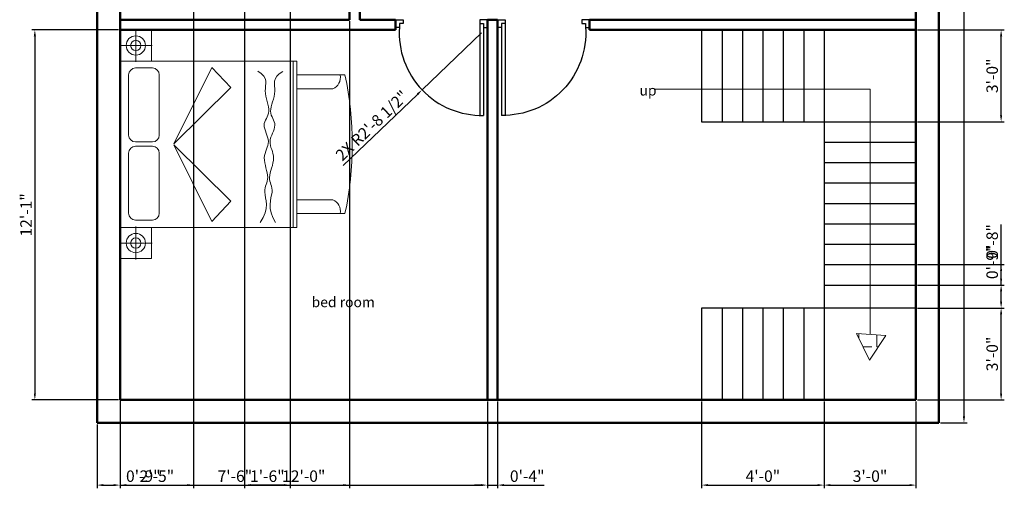
# Model space of a CAD drawing. Units: inches. Extents: x 1253 to 1645, y 2180 to 2698.
# Tile 1 of 5: x 1257 to 1643, y 2180 to 2363. Entities that reach past the tile are written whole.
import ezdxf

# ---------------------------------------------------------------- set-up
doc = ezdxf.new("R2010")
doc.units = ezdxf.units.IN
for name, color, linetype, lineweight in [('A-ANNO-DIMS', 2, 'Continuous', 18), ('A-ANNO-SYMB', 7, 'Continuous', 18), ('A-ANNO-TEXT', 7, 'Continuous', 18), ('A-AREA-IDEN', 7, 'Continuous', 25), ('A-DOOR', 4, 'Continuous', 25), ('A-FLOR-STRS', 7, 'Continuous', 25), ('A-FURN', 8, 'Continuous', 18), ('wall', 7, 'Continuous', 50)]:
    doc.layers.add(name, color=color, linetype=linetype, lineweight=lineweight)
doc.styles.get("Standard").update_dxf_attribs({"font": 'arial.ttf'})
doc.dimstyles.new('ISO-25', dxfattribs={"dimtxt": 4.5, "dimasz": 2.5, "dimexe": 1.25, "dimexo": 0.625, "dimtad": 1, "dimdec": 1, "dimlunit": 3, "dimtxsty": 'Standard', "dimcen": 4.5, "dimadec": 0, "dimazin": 0, "dimtfac": 1, "dimtdec": 1, "dimtmove": 0, "dimatfit": 3, "dimfxl": 1, "dimarcsym": 0})

# ---------------------------------------------------------------- blocks, each defined once
blk = doc.blocks.new('A$C4F543DC7')
for p, q in [((0.013, 3.35, -0.169), (3.313, 3.35, -0.169)), ((0.463, 3.35, -0.169), (0.013, 3.35, -0.169)), ((0.013, 2.896, -0.169), (0.013, 3.35, -0.169)), ((0.013, 3.35, -0.169), (0.013, 2.896, -0.169)), ((0.238, 3.123, -0.439), (0.238, 3.361, -0.439)), ((0.463, 3.35, -0.169), (0.463, 0.8, -0.169)), ((2.863, 3.35, -0.169), (0.463, 3.35, -0.169)), ((0.463, 2.896, -0.169), (0.463, 3.35, -0.169)), ((2.863, 0.8, -0.169), (2.863, 3.35, -0.169)), ((2.863, 3.35, -0.169), (3.313, 3.35, -0.169)), ((2.863, 2.896, -0.169), (2.863, 3.35, -0.169)), ((3.089, 3.123, -0.439), (3.089, 3.361, -0.439)), ((3.313, 3.35, -0.169), (3.313, 2.896, -0.169)), ((3.313, 3.35, -0.169), (3.313, 2.896, -0.169)), ((1.535, 3.226, -0.169), (0.668, 3.226, -0.169)), ((2.664, 3.226, -0.169), (1.797, 3.226, -0.169)), ((0.238, 3.123, -0.439), (0, 3.123, -0.439)), ((0.238, 3.123, -0.439), (0.476, 3.123, -0.439)), ((0.238, 3.123, -0.439), (0.238, 2.885, -0.439)), ((0.568, 3.126, -0.169), (0.568, 2.884, -0.169)), ((1.635, 2.884, -0.169), (1.635, 3.126, -0.169)), ((1.697, 3.126, -0.169), (1.697, 2.884, -0.169)), ((2.764, 2.884, -0.169), (2.764, 3.126, -0.169)), ((3.089, 3.123, -0.439), (2.851, 3.123, -0.439)), ((3.089, 3.123, -0.439), (3.089, 2.885, -0.439)), ((3.089, 3.123, -0.439), (3.327, 3.123, -0.439)), ((0.463, 2.896, -0.169), (0.013, 2.896, -0.169)), ((0.013, 2.896, -0.169), (0.463, 2.896, -0.169)), ((0.463, 0.8, -0.169), (0.463, 2.896, -0.169)), ((2.863, 2.896, -0.169), (2.863, 0.8, -0.169)), ((3.313, 2.896, -0.169), (2.863, 2.896, -0.169)), ((3.313, 2.896, -0.169), (2.863, 2.896, -0.169)), ((0.668, 2.784, -0.169), (1.535, 2.784, -0.169)), ((1.797, 2.784, -0.169), (2.664, 2.784, -0.169)), ((1.653, 2.573, -0.169), (0.55, 2.025, -0.169)), ((0.841, 1.752, -0.169), (1.653, 2.573, -0.169)), ((2.481, 1.752, -0.169), (1.669, 2.573, -0.169)), ((1.669, 2.573, -0.169), (2.772, 2.025, -0.169)), ((0.55, 2.025, -0.169), (0.841, 1.752, -0.169)), ((2.772, 2.025, -0.169), (2.481, 1.752, -0.169)), ((0.537, 1.327, -0.169), (0.609, 1.284, -0.169)), ((0.609, 1.284, -0.169), (0.676, 1.257, -0.169)), ((2.648, 1.277, -0.169), (2.683, 1.312, -0.169)), ((2.683, 1.312, -0.169), (2.718, 1.364, -0.169)), ((0.533, 1.105, -0.169), (0.607, 1.146, -0.169)), ((0.607, 1.146, -0.169), (0.674, 1.171, -0.169)), ((0.674, 1.171, -0.169), (0.736, 1.183, -0.169)), ((0.676, 1.257, -0.169), (0.737, 1.243, -0.169)), ((0.736, 1.183, -0.169), (0.793, 1.185, -0.169)), ((0.737, 1.243, -0.169), (0.794, 1.239, -0.169)), ((0.793, 1.185, -0.169), (0.845, 1.18, -0.169)), ((0.794, 1.239, -0.169), (0.846, 1.242, -0.169)), ((0.845, 1.18, -0.169), (0.891, 1.172, -0.169)), ((0.846, 1.242, -0.169), (0.893, 1.249, -0.169)), ((0.891, 1.172, -0.169), (0.933, 1.163, -0.169)), ((0.893, 1.249, -0.169), (0.935, 1.256, -0.169)), ((0.933, 1.163, -0.169), (0.97, 1.156, -0.169)), ((0.935, 1.256, -0.169), (0.972, 1.261, -0.169)), ((0.97, 1.156, -0.169), (1.003, 1.155, -0.169)), ((0.972, 1.261, -0.169), (1.004, 1.262, -0.169)), ((1.003, 1.155, -0.169), (1.032, 1.158, -0.169)), ((1.004, 1.262, -0.169), (1.033, 1.258, -0.169)), ((1.032, 1.158, -0.169), (1.058, 1.164, -0.169)), ((1.033, 1.258, -0.169), (1.06, 1.251, -0.169)), ((1.058, 1.164, -0.169), (1.083, 1.172, -0.169)), ((1.06, 1.251, -0.169), (1.084, 1.242, -0.169)), ((1.083, 1.172, -0.169), (1.107, 1.18, -0.169)), ((1.084, 1.242, -0.169), (1.108, 1.234, -0.169)), ((1.107, 1.18, -0.169), (1.132, 1.187, -0.169)), ((1.108, 1.234, -0.169), (1.132, 1.226, -0.169)), ((1.132, 1.226, -0.169), (1.158, 1.22, -0.169)), ((1.132, 1.187, -0.169), (1.157, 1.192, -0.169)), ((1.157, 1.192, -0.169), (1.185, 1.193, -0.169)), ((1.158, 1.22, -0.169), (1.185, 1.218, -0.169)), ((1.185, 1.218, -0.169), (1.216, 1.22, -0.169)), ((1.185, 1.193, -0.169), (1.216, 1.19, -0.169)), ((1.216, 1.22, -0.169), (1.25, 1.226, -0.169)), ((1.216, 1.19, -0.169), (1.249, 1.183, -0.169)), ((1.249, 1.183, -0.169), (1.284, 1.173, -0.169)), ((1.25, 1.226, -0.169), (1.285, 1.235, -0.169)), ((1.284, 1.173, -0.169), (1.321, 1.163, -0.169)), ((1.285, 1.235, -0.169), (1.322, 1.244, -0.169)), ((1.321, 1.163, -0.169), (1.358, 1.152, -0.169)), ((1.322, 1.244, -0.169), (1.359, 1.253, -0.169)), ((1.358, 1.152, -0.169), (1.394, 1.143, -0.169)), ((1.359, 1.253, -0.169), (1.396, 1.261, -0.169)), ((1.394, 1.143, -0.169), (1.431, 1.137, -0.169)), ((1.396, 1.261, -0.169), (1.433, 1.266, -0.169)), ((1.431, 1.137, -0.169), (1.466, 1.135, -0.169)), ((1.433, 1.266, -0.169), (1.468, 1.268, -0.169)), ((1.466, 1.135, -0.169), (1.499, 1.137, -0.169)), ((1.468, 1.268, -0.169), (1.501, 1.264, -0.169)), ((1.499, 1.137, -0.169), (1.531, 1.143, -0.169)), ((1.501, 1.264, -0.169), (1.532, 1.257, -0.169)), ((1.531, 1.143, -0.169), (1.561, 1.152, -0.169)), ((1.532, 1.257, -0.169), (1.562, 1.247, -0.169)), ((1.561, 1.152, -0.169), (1.59, 1.162, -0.169)), ((1.562, 1.247, -0.169), (1.591, 1.237, -0.169)), ((1.59, 1.162, -0.169), (1.619, 1.172, -0.169)), ((1.591, 1.237, -0.169), (1.62, 1.226, -0.169)), ((1.619, 1.172, -0.169), (1.648, 1.18, -0.169)), ((1.62, 1.226, -0.169), (1.648, 1.217, -0.169)), ((1.648, 1.217, -0.169), (1.676, 1.211, -0.169)), ((1.648, 1.18, -0.169), (1.676, 1.185, -0.169)), ((1.676, 1.211, -0.169), (1.705, 1.209, -0.169)), ((1.676, 1.185, -0.169), (1.705, 1.186, -0.169)), ((1.705, 1.209, -0.169), (1.735, 1.212, -0.169)), ((1.705, 1.186, -0.169), (1.734, 1.182, -0.169)), ((1.734, 1.182, -0.169), (1.764, 1.173, -0.169)), ((1.735, 1.212, -0.169), (1.765, 1.22, -0.169)), ((1.764, 1.173, -0.169), (1.794, 1.162, -0.169)), ((1.765, 1.22, -0.169), (1.795, 1.23, -0.169)), ((1.794, 1.162, -0.169), (1.824, 1.149, -0.169)), ((1.795, 1.23, -0.169), (1.826, 1.242, -0.169)), ((1.824, 1.149, -0.169), (1.854, 1.137, -0.169)), ((1.826, 1.242, -0.169), (1.856, 1.253, -0.169)), ((1.854, 1.137, -0.169), (1.883, 1.126, -0.169)), ((1.856, 1.253, -0.169), (1.885, 1.263, -0.169)), ((1.885, 1.263, -0.169), (1.913, 1.27, -0.169)), ((1.913, 1.27, -0.169), (1.94, 1.272, -0.169)), ((1.94, 1.272, -0.169), (1.965, 1.269, -0.169)), ((1.965, 1.269, -0.169), (1.989, 1.262, -0.169)), ((1.989, 1.262, -0.169), (2.012, 1.251, -0.169)), ((2.011, 1.134, -0.169), (2.034, 1.145, -0.169)), ((2.012, 1.251, -0.169), (2.036, 1.239, -0.169)), ((2.034, 1.145, -0.169), (2.059, 1.157, -0.169)), ((2.036, 1.239, -0.169), (2.06, 1.227, -0.169)), ((2.059, 1.157, -0.169), (2.084, 1.167, -0.169)), ((2.06, 1.227, -0.169), (2.085, 1.216, -0.169)), ((2.084, 1.167, -0.169), (2.111, 1.174, -0.169)), ((2.085, 1.216, -0.169), (2.112, 1.208, -0.169)), ((2.111, 1.174, -0.169), (2.14, 1.177, -0.169)), ((2.112, 1.208, -0.169), (2.141, 1.204, -0.169)), ((2.14, 1.177, -0.169), (2.172, 1.175, -0.169)), ((2.141, 1.204, -0.169), (2.172, 1.205, -0.169)), ((2.172, 1.205, -0.169), (2.206, 1.21, -0.169)), ((2.172, 1.175, -0.169), (2.206, 1.169, -0.169)), ((2.206, 1.21, -0.169), (2.242, 1.218, -0.169)), ((2.206, 1.169, -0.169), (2.241, 1.16, -0.169)), ((2.241, 1.16, -0.169), (2.278, 1.149, -0.169)), ((2.242, 1.218, -0.169), (2.279, 1.228, -0.169)), ((2.278, 1.149, -0.169), (2.316, 1.138, -0.169)), ((2.279, 1.228, -0.169), (2.317, 1.238, -0.169)), ((2.316, 1.138, -0.169), (2.354, 1.128, -0.169)), ((2.317, 1.238, -0.169), (2.356, 1.246, -0.169)), ((2.356, 1.246, -0.169), (2.394, 1.253, -0.169)), ((2.394, 1.253, -0.169), (2.433, 1.255, -0.169)), ((2.433, 1.255, -0.169), (2.47, 1.253, -0.169)), ((2.47, 1.253, -0.169), (2.506, 1.249, -0.169)), ((2.506, 1.249, -0.169), (2.542, 1.246, -0.169)), ((2.542, 1.246, -0.169), (2.578, 1.248, -0.169)), ((2.578, 1.248, -0.169), (2.613, 1.257, -0.169)), ((2.613, 1.257, -0.169), (2.648, 1.277, -0.169)), ((1.883, 1.126, -0.169), (1.911, 1.119, -0.169)), ((1.911, 1.119, -0.169), (1.937, 1.115, -0.169)), ((1.937, 1.115, -0.169), (1.963, 1.118, -0.169)), ((1.963, 1.118, -0.169), (1.987, 1.124, -0.169)), ((1.987, 1.124, -0.169), (2.011, 1.134, -0.169)), ((2.354, 1.128, -0.169), (2.392, 1.121, -0.169)), ((2.392, 1.121, -0.169), (2.43, 1.117, -0.169)), ((2.43, 1.117, -0.169), (2.468, 1.118, -0.169)), ((2.468, 1.118, -0.169), (2.504, 1.121, -0.169)), ((2.504, 1.121, -0.169), (2.54, 1.123, -0.169)), ((2.54, 1.123, -0.169), (2.576, 1.12, -0.169)), ((2.576, 1.12, -0.169), (2.611, 1.109, -0.169)), ((2.611, 1.109, -0.169), (2.645, 1.088, -0.169)), ((2.645, 1.088, -0.169), (2.679, 1.052, -0.169)), ((2.679, 1.052, -0.169), (2.712, 0.999, -0.169)), ((0.463, 0.85, -0.169), (2.863, 0.85, -0.169)), ((0.463, 0.8, -0.169), (2.863, 0.8, -0.169)), ((0.663, 0.8, -0.169), (0.463, 0.8, -0.169)), ((0.663, 0.8, -0.169), (2.663, 0.8, -0.169)), ((0.663, 0.104, -0.169), (0.663, 0.8, -0.169)), ((0.663, 0.104, -0.169), (0.663, 0.8, -0.169)), ((0.863, 0.281, -0.169), (0.863, 0.8, -0.169)), ((2.463, 0.8, -0.169), (2.463, 0.281, -0.169)), ((2.863, 0.8, -0.169), (2.663, 0.8, -0.169)), ((2.663, 0.8, -0.169), (2.663, 0.104, -0.169)), ((2.663, 0.8, -0.169), (2.663, 0.104, -0.169))]:
    blk.add_line(p, q)
for centre, radius in [((0.238, 3.123, -0.439), 0.139), ((0.238, 3.123, -0.439), 0.075), ((3.089, 3.123, -0.439), 0.139), ((3.089, 3.123, -0.439), 0.075)]:
    blk.add_circle(centre, radius)
for centre, radius, start, end in [((0.668, 3.126, -0.169), 0.1, 90, 180), ((1.535, 3.126, -0.169), 0.1, 0, 90), ((1.797, 3.126, -0.169), 0.1, 90, 180), ((2.664, 3.126, -0.169), 0.1, 0, 90), ((0.668, 2.884, -0.169), 0.1, 180, 270), ((1.535, 2.884, -0.169), 0.1, 270, 0), ((1.797, 2.884, -0.169), 0.1, 180, 270), ((2.664, 2.884, -0.169), 0.1, 270, 0), ((0.699, 0.347, -0.169), 0.177, 258.2616, 338.032), ((2.627, 0.347, -0.169), 0.177, 201.968, 281.7384), ((1.663, 4.86, -0.169), 4.86, 258.1252, 281.8748), ((1.663, 4.86, -0.169), 4.86, 258.1252, 281.8748)]:
    blk.add_arc(centre, radius, start, end)
blk = doc.blocks.new('*D14')
at = {"layer": 'A-ANNO-DIMS', "color": 0, "lineweight": -2, "transparency": 16777216}
for p, q in [((1617.57, 2667.35), (1628.02, 2667.35)), ((1626.77, 2664.85), (1626.77, 2207.85)), ((1617.57, 2205.35), (1628.02, 2205.35))]:
    blk.add_line(p, q, dxfattribs=at)
at = {"layer": 'A-ANNO-DIMS', "color": 0, "transparency": 16777216}
for points in [[(1626.36, 2664.85), (1627.19, 2664.85), (1626.77, 2667.35)], [(1626.36, 2207.85), (1627.19, 2207.85), (1626.77, 2205.35)]]:
    blk.add_solid(points, dxfattribs=at)
at = {"layer": 'Defpoints', "color": 0, "transparency": 16777216}
for p in [(1616.94, 2667.35), (1616.94, 2205.35), (1626.77, 2205.35)]:
    blk.add_point(p, dxfattribs=at)
at = {"layer": 'A-ANNO-DIMS', "color": 0, "transparency": 16777216, "insert": (1623.85, 2436.35), "char_height": 4.5, "attachment_point": 5, "rotation": 90}
blk.add_mtext('38\'-6"', dxfattribs=at)
blk = doc.blocks.new('DOOR-SWING-36IN')
for p, q in [((1.5, 1.5), (1.5, 37.5)), ((3, 1.5), (3, 37.5)), ((0, 3), (0, 0)), ((1.5, 3), (0, 3)), ((1.5, 1.5), (1.5, 3)), ((3, 1.5), (1.5, 1.5)), ((3, 0), (3, 1.5)), ((33, 0), (33, 1.5)), ((33, 1.5), (34.5, 1.5)), ((34.5, 1.5), (34.5, 3)), ((34.5, 3), (36, 3)), ((36, 3), (36, 0)), ((0, 0), (3, 0)), ((36, 0), (33, 0))]:
    blk.add_line(p, q)
blk.add_arc((2.25, 5.18), 32.32, 356.1244, 91.3295)
blk = doc.blocks.new('*D33')
at = {"layer": 'A-ANNO-DIMS', "color": 0, "lineweight": -2, "transparency": 16777216}
for p, q in [((1295.32, 2359.35), (1261.29, 2359.35)), ((1262.54, 2356.85), (1262.54, 2216.85)), ((1295.32, 2214.35), (1261.29, 2214.35))]:
    blk.add_line(p, q, dxfattribs=at)
at = {"layer": 'A-ANNO-DIMS', "color": 0, "transparency": 16777216}
for points in [[(1262.12, 2356.85), (1262.96, 2356.85), (1262.54, 2359.35)], [(1262.12, 2216.85), (1262.96, 2216.85), (1262.54, 2214.35)]]:
    blk.add_solid(points, dxfattribs=at)
at = {"layer": 'Defpoints', "color": 0, "transparency": 16777216}
for p in [(1295.94, 2359.35), (1262.54, 2214.35), (1295.94, 2214.35)]:
    blk.add_point(p, dxfattribs=at)
at = {"layer": 'A-ANNO-DIMS', "color": 0, "transparency": 16777216, "insert": (1259.66, 2286.85), "char_height": 4.5, "attachment_point": 5, "rotation": 90}
blk.add_mtext('12\'-1"', dxfattribs=at)
blk = doc.blocks.new('*D34')
at = {"layer": 'A-ANNO-DIMS', "color": 0, "lineweight": -2, "transparency": 16777216}
for p, q in [((1295.94, 2213.72), (1295.94, 2179.7)), ((1439.94, 2213.72), (1439.94, 2179.7)), ((1298.44, 2180.95), (1437.44, 2180.95))]:
    blk.add_line(p, q, dxfattribs=at)
at = {"layer": 'A-ANNO-DIMS', "color": 0, "transparency": 16777216}
for points in [[(1298.44, 2181.36), (1298.44, 2180.53), (1295.94, 2180.95)], [(1437.44, 2181.36), (1437.44, 2180.53), (1439.94, 2180.95)]]:
    blk.add_solid(points, dxfattribs=at)
at = {"layer": 'Defpoints', "color": 0, "transparency": 16777216}
for p in [(1295.94, 2214.35), (1439.94, 2214.35), (1439.94, 2180.95)]:
    blk.add_point(p, dxfattribs=at)
at = {"layer": 'A-ANNO-DIMS', "color": 0, "transparency": 16777216, "insert": (1367.94, 2183.87), "char_height": 4.5, "attachment_point": 5}
blk.add_mtext('12\'-0"', dxfattribs=at)
blk = doc.blocks.new('*D35')
at = {"layer": 'A-ANNO-DIMS', "color": 0, "lineweight": -2, "transparency": 16777216}
for p, q in [((1295.94, 2362.72), (1295.94, 2179.7)), ((1385.94, 2362.72), (1385.94, 2179.7)), ((1298.44, 2180.95), (1383.44, 2180.95))]:
    blk.add_line(p, q, dxfattribs=at)
at = {"layer": 'A-ANNO-DIMS', "color": 0, "transparency": 16777216}
for points in [[(1298.44, 2181.36), (1298.44, 2180.53), (1295.94, 2180.95)], [(1383.44, 2181.36), (1383.44, 2180.53), (1385.94, 2180.95)]]:
    blk.add_solid(points, dxfattribs=at)
at = {"layer": 'Defpoints', "color": 0, "transparency": 16777216}
for p in [(1295.94, 2363.35), (1385.94, 2363.35), (1385.94, 2180.95)]:
    blk.add_point(p, dxfattribs=at)
at = {"layer": 'A-ANNO-DIMS', "color": 0, "transparency": 16777216, "insert": (1340.94, 2183.87), "char_height": 4.5, "attachment_point": 5}
blk.add_mtext('7\'-6"', dxfattribs=at)
blk = doc.blocks.new('*D36')
at = {"layer": 'A-ANNO-DIMS', "color": 0, "lineweight": -2, "transparency": 16777216}
for p, q in [((1523.94, 2213.72), (1523.94, 2179.7)), ((1571.94, 2213.72), (1571.94, 2179.7)), ((1526.44, 2180.95), (1569.44, 2180.95))]:
    blk.add_line(p, q, dxfattribs=at)
at = {"layer": 'A-ANNO-DIMS', "color": 0, "transparency": 16777216}
for points in [[(1526.44, 2181.36), (1526.44, 2180.53), (1523.94, 2180.95)], [(1569.44, 2181.36), (1569.44, 2180.53), (1571.94, 2180.95)]]:
    blk.add_solid(points, dxfattribs=at)
at = {"layer": 'Defpoints', "color": 0, "transparency": 16777216}
for p in [(1523.94, 2214.35), (1571.94, 2214.35), (1571.94, 2180.95)]:
    blk.add_point(p, dxfattribs=at)
at = {"layer": 'A-ANNO-DIMS', "color": 0, "transparency": 16777216, "insert": (1547.94, 2183.87), "char_height": 4.5, "attachment_point": 5}
blk.add_mtext('4\'-0"', dxfattribs=at)
blk = doc.blocks.new('*D37')
at = {"layer": 'A-ANNO-DIMS', "color": 0, "lineweight": -2, "transparency": 16777216}
for p, q in [((1571.94, 2213.72), (1571.94, 2179.7)), ((1607.94, 2213.72), (1607.94, 2179.7)), ((1574.44, 2180.95), (1605.44, 2180.95))]:
    blk.add_line(p, q, dxfattribs=at)
at = {"layer": 'A-ANNO-DIMS', "color": 0, "transparency": 16777216}
for points in [[(1574.44, 2181.36), (1574.44, 2180.53), (1571.94, 2180.95)], [(1605.44, 2181.36), (1605.44, 2180.53), (1607.94, 2180.95)]]:
    blk.add_solid(points, dxfattribs=at)
at = {"layer": 'Defpoints', "color": 0, "transparency": 16777216}
for p in [(1571.94, 2214.35), (1607.94, 2214.35), (1607.94, 2180.95)]:
    blk.add_point(p, dxfattribs=at)
at = {"layer": 'A-ANNO-DIMS', "color": 0, "transparency": 16777216, "insert": (1589.94, 2183.87), "char_height": 4.5, "attachment_point": 5}
blk.add_mtext('3\'-0"', dxfattribs=at)
blk = doc.blocks.new('*D38')
at = {"layer": 'A-ANNO-DIMS', "color": 0, "lineweight": -2, "transparency": 16777216}
for p, q in [((1641.34, 2259.35), (1641.34, 2275.06)), ((1608.57, 2259.35), (1642.59, 2259.35)), ((1641.34, 2252.85), (1641.34, 2256.85)), ((1608.57, 2250.35), (1642.59, 2250.35))]:
    blk.add_line(p, q, dxfattribs=at)
at = {"layer": 'A-ANNO-DIMS', "color": 0, "transparency": 16777216}
for points in [[(1640.92, 2256.85), (1641.76, 2256.85), (1641.34, 2259.35)], [(1640.92, 2252.85), (1641.76, 2252.85), (1641.34, 2250.35)]]:
    blk.add_solid(points, dxfattribs=at)
at = {"layer": 'Defpoints', "color": 0, "transparency": 16777216}
for p in [(1607.94, 2259.35), (1641.34, 2259.35), (1607.94, 2250.35)]:
    blk.add_point(p, dxfattribs=at)
at = {"layer": 'A-ANNO-DIMS', "color": 0, "transparency": 16777216, "insert": (1638.42, 2268.45), "char_height": 4.5, "attachment_point": 5, "rotation": 90}
blk.add_mtext('0\'-9"', dxfattribs=at)
blk = doc.blocks.new('*D39')
at = {"layer": 'A-ANNO-DIMS', "color": 0, "lineweight": -2, "transparency": 16777216}
for p, q in [((1641.34, 2267.35), (1641.34, 2283.06)), ((1608.57, 2267.35), (1642.59, 2267.35)), ((1641.34, 2261.85), (1641.34, 2264.85)), ((1608.57, 2259.35), (1642.59, 2259.35))]:
    blk.add_line(p, q, dxfattribs=at)
at = {"layer": 'A-ANNO-DIMS', "color": 0, "transparency": 16777216}
for points in [[(1640.92, 2264.85), (1641.76, 2264.85), (1641.34, 2267.35)], [(1640.92, 2261.85), (1641.76, 2261.85), (1641.34, 2259.35)]]:
    blk.add_solid(points, dxfattribs=at)
at = {"layer": 'Defpoints', "color": 0, "transparency": 16777216}
for p in [(1607.94, 2267.35), (1641.34, 2267.35), (1607.94, 2259.35)]:
    blk.add_point(p, dxfattribs=at)
at = {"layer": 'A-ANNO-DIMS', "color": 0, "transparency": 16777216, "insert": (1638.42, 2276.45), "char_height": 4.5, "attachment_point": 5, "rotation": 90}
blk.add_mtext('0\'-8"', dxfattribs=at)
blk = doc.blocks.new('*D40')
at = {"layer": 'A-ANNO-DIMS', "color": 0, "lineweight": -2, "transparency": 16777216}
for p, q in [((1608.57, 2359.35), (1642.59, 2359.35)), ((1641.34, 2325.85), (1641.34, 2356.85)), ((1608.57, 2323.35), (1642.59, 2323.35))]:
    blk.add_line(p, q, dxfattribs=at)
at = {"layer": 'A-ANNO-DIMS', "color": 0, "transparency": 16777216}
for points in [[(1640.92, 2356.85), (1641.76, 2356.85), (1641.34, 2359.35)], [(1640.92, 2325.85), (1641.76, 2325.85), (1641.34, 2323.35)]]:
    blk.add_solid(points, dxfattribs=at)
at = {"layer": 'Defpoints', "color": 0, "transparency": 16777216}
for p in [(1607.94, 2359.35), (1641.34, 2359.35), (1607.94, 2323.35)]:
    blk.add_point(p, dxfattribs=at)
at = {"layer": 'A-ANNO-DIMS', "color": 0, "transparency": 16777216, "insert": (1638.42, 2341.35), "char_height": 4.5, "attachment_point": 5, "rotation": 90}
blk.add_mtext('3\'-0"', dxfattribs=at)
blk = doc.blocks.new('*D41')
at = {"layer": 'A-ANNO-DIMS', "color": 0, "lineweight": -2, "transparency": 16777216}
for p, q in [((1608.57, 2250.35), (1642.59, 2250.35)), ((1641.34, 2216.85), (1641.34, 2247.85)), ((1608.57, 2214.35), (1642.59, 2214.35))]:
    blk.add_line(p, q, dxfattribs=at)
at = {"layer": 'A-ANNO-DIMS', "color": 0, "transparency": 16777216}
for points in [[(1640.92, 2247.85), (1641.76, 2247.85), (1641.34, 2250.35)], [(1640.92, 2216.85), (1641.76, 2216.85), (1641.34, 2214.35)]]:
    blk.add_solid(points, dxfattribs=at)
at = {"layer": 'Defpoints', "color": 0, "transparency": 16777216}
for p in [(1607.94, 2250.35), (1641.34, 2250.35), (1607.94, 2214.35)]:
    blk.add_point(p, dxfattribs=at)
at = {"layer": 'A-ANNO-DIMS', "color": 0, "transparency": 16777216, "insert": (1638.42, 2232.35), "char_height": 4.5, "attachment_point": 5, "rotation": 90}
blk.add_mtext('3\'-0"', dxfattribs=at)
blk = doc.blocks.new('*D42')
at = {"layer": 'A-ANNO-DIMS', "color": 0, "lineweight": -2, "transparency": 16777216}
for p, q in [((1295.94, 2213.72), (1295.94, 2179.7)), ((1286.94, 2204.72), (1286.94, 2179.7)), ((1289.44, 2180.95), (1293.44, 2180.95)), ((1295.94, 2180.95), (1311.65, 2180.95))]:
    blk.add_line(p, q, dxfattribs=at)
at = {"layer": 'A-ANNO-DIMS', "color": 0, "transparency": 16777216}
for points in [[(1289.44, 2181.36), (1289.44, 2180.53), (1286.94, 2180.95)], [(1293.44, 2181.36), (1293.44, 2180.53), (1295.94, 2180.95)]]:
    blk.add_solid(points, dxfattribs=at)
at = {"layer": 'Defpoints', "color": 0, "transparency": 16777216}
for p in [(1295.94, 2214.35), (1286.94, 2205.35), (1295.94, 2180.95)]:
    blk.add_point(p, dxfattribs=at)
at = {"layer": 'A-ANNO-DIMS', "color": 0, "transparency": 16777216, "insert": (1305.05, 2183.87), "char_height": 4.5, "attachment_point": 5}
blk.add_mtext('0\'-9"', dxfattribs=at)
blk = doc.blocks.new('*D43')
at = {"layer": 'A-ANNO-DIMS', "color": 0, "lineweight": -2, "transparency": 16777216}
for p, q in [((1439.94, 2213.72), (1439.94, 2179.7)), ((1443.94, 2213.72), (1443.94, 2179.7)), ((1437.44, 2180.95), (1434.94, 2180.95)), ((1439.94, 2180.95), (1443.94, 2180.95)), ((1446.44, 2180.95), (1462.15, 2180.95))]:
    blk.add_line(p, q, dxfattribs=at)
at = {"layer": 'A-ANNO-DIMS', "color": 0, "transparency": 16777216}
for points in [[(1437.44, 2181.36), (1437.44, 2180.53), (1439.94, 2180.95)], [(1446.44, 2181.36), (1446.44, 2180.53), (1443.94, 2180.95)]]:
    blk.add_solid(points, dxfattribs=at)
at = {"layer": 'Defpoints', "color": 0, "transparency": 16777216}
for p in [(1439.94, 2214.35), (1443.94, 2214.35), (1443.94, 2180.95)]:
    blk.add_point(p, dxfattribs=at)
at = {"layer": 'A-ANNO-DIMS', "color": 0, "transparency": 16777216, "insert": (1455.55, 2183.87), "char_height": 4.5, "attachment_point": 5}
blk.add_mtext('0\'-4"', dxfattribs=at)
blk = doc.blocks.new('*D48')
at = {"layer": 'A-ANNO-DIMS', "color": 0, "lineweight": -2, "transparency": 16777216}
for p, q in [((1295.94, 2396.31), (1295.94, 2179.7)), ((1324.77, 2396.41), (1324.77, 2179.7)), ((1298.44, 2180.95), (1322.27, 2180.95))]:
    blk.add_line(p, q, dxfattribs=at)
at = {"layer": 'A-ANNO-DIMS', "color": 0, "transparency": 16777216}
for points in [[(1298.44, 2181.36), (1298.44, 2180.53), (1295.94, 2180.95)], [(1322.27, 2181.36), (1322.27, 2180.53), (1324.77, 2180.95)]]:
    blk.add_solid(points, dxfattribs=at)
at = {"layer": 'Defpoints', "color": 0, "transparency": 16777216}
for p in [(1295.94, 2396.94), (1324.77, 2397.03), (1324.77, 2180.95)]:
    blk.add_point(p, dxfattribs=at)
at = {"layer": 'A-ANNO-DIMS', "color": 0, "transparency": 16777216, "insert": (1310.36, 2183.87), "char_height": 4.5, "attachment_point": 5}
blk.add_mtext('2\'-5"', dxfattribs=at)
blk = doc.blocks.new('*D52')
at = {"layer": 'A-ANNO-DIMS', "color": 0, "lineweight": -2, "transparency": 16777216}
for p, q in [((1344.68, 2396.41), (1344.68, 2179.7)), ((1362.68, 2396.31), (1362.68, 2179.7)), ((1360.18, 2180.95), (1347.18, 2180.95))]:
    blk.add_line(p, q, dxfattribs=at)
at = {"layer": 'A-ANNO-DIMS', "color": 0, "transparency": 16777216}
for points in [[(1347.18, 2181.36), (1347.18, 2180.53), (1344.68, 2180.95)], [(1360.18, 2181.36), (1360.18, 2180.53), (1362.68, 2180.95)]]:
    blk.add_solid(points, dxfattribs=at)
at = {"layer": 'Defpoints', "color": 0, "transparency": 16777216}
for p in [(1344.68, 2397.03), (1362.68, 2396.94), (1344.68, 2180.95)]:
    blk.add_point(p, dxfattribs=at)
at = {"layer": 'A-ANNO-DIMS', "color": 0, "transparency": 16777216, "insert": (1353.68, 2183.87), "char_height": 4.5, "attachment_point": 5}
blk.add_mtext('1\'-6"', dxfattribs=at)
blk = doc.blocks.new('*D60')
at = {"layer": 'A-ANNO-DIMS', "color": 0, "lineweight": -2, "transparency": 16777216}
for p, q in [((1437.69, 2358.16), (1414.33, 2335.82)), ((1383.44, 2306.27), (1412.53, 2334.09))]:
    blk.add_line(p, q, dxfattribs=at)
at = {"layer": 'A-ANNO-DIMS', "color": 0, "transparency": 16777216}
blk.add_solid([(1412.24, 2334.39), (1412.81, 2333.79), (1414.33, 2335.82)], dxfattribs=at)
at = {"layer": 'Defpoints', "color": 0, "transparency": 16777216}
for p in [(1437.69, 2358.16), (1414.33, 2335.82)]:
    blk.add_point(p, dxfattribs=at)
at = {"layer": 'A-ANNO-DIMS', "color": 0, "transparency": 16777216, "insert": (1395.04, 2321.45), "char_height": 4.5, "attachment_point": 5, "rotation": 43.7269}
blk.add_mtext('2X R2\'-8 1/2"', dxfattribs=at)

msp = doc.modelspace()

# ---------------------------------------------------------------- hatches: boundary and pattern name
at = {"layer": 'A-ANNO-SYMB'}
h = msp.add_hatch(dxfattribs=at)
h.set_pattern_fill('ANGLE', color=256)
h.set_pattern_definition([(0, (0, 0), (0, 6.985), [5.08, -1.905]), (90, (0, 0), (-6.985, 4e-16), [5.08, -1.905])])
h.paths.add_polyline_path([(1596.21, 2239.56), (1584.68, 2240.33), (1589.78, 2229.95)])

# ---------------------------------------------------------------- linework, layer by layer
for p, q in [((1505.72, 2336.08), (1589.94, 2336.08)), ((1589.94, 2336.08), (1589.94, 2240.18))]:
    msp.add_line(p, q, dxfattribs=at)
msp.add_lwpolyline([(1589.78, 2229.95), (1596.21, 2239.56), (1584.68, 2240.33)], close=True, dxfattribs=at)
at = {"layer": 'A-FLOR-STRS'}
for p, q in [((1523.94, 2359.35), (1523.94, 2323.35)), ((1531.94, 2359.35), (1531.94, 2323.35)), ((1539.94, 2359.35), (1539.94, 2323.35)), ((1547.94, 2359.35), (1547.94, 2323.35)), ((1555.94, 2359.35), (1555.94, 2323.35)), ((1563.94, 2359.35), (1563.94, 2323.35)), ((1607.94, 2359.35), (1571.94, 2359.35)), ((1571.94, 2359.35), (1571.94, 2323.35)), ((1607.94, 2323.35), (1607.94, 2359.35)), ((1523.94, 2323.35), (1571.94, 2323.35)), ((1571.94, 2323.35), (1607.94, 2323.35)), ((1571.94, 2323.35), (1571.94, 2250.35)), ((1571.94, 2315.35), (1607.94, 2315.35)), ((1571.94, 2307.35), (1607.94, 2307.35)), ((1571.94, 2299.35), (1607.94, 2299.35)), ((1571.94, 2291.35), (1607.94, 2291.35)), ((1571.94, 2283.35), (1607.94, 2283.35)), ((1571.94, 2275.35), (1607.94, 2275.35)), ((1571.94, 2267.35), (1607.94, 2267.35)), ((1571.94, 2259.35), (1607.94, 2259.35)), ((1523.94, 2250.35), (1523.94, 2214.35)), ((1571.94, 2250.35), (1523.94, 2250.35)), ((1531.94, 2250.35), (1531.94, 2214.35)), ((1539.94, 2250.35), (1539.94, 2214.35)), ((1547.94, 2250.35), (1547.94, 2214.35)), ((1555.94, 2250.35), (1555.94, 2214.35)), ((1563.94, 2250.35), (1563.94, 2214.35)), ((1607.94, 2250.35), (1571.94, 2250.35)), ((1571.94, 2250.35), (1571.94, 2214.35)), ((1607.94, 2214.35), (1607.94, 2250.35)), ((1571.94, 2214.35), (1607.94, 2214.35))]:
    msp.add_line(p, q, dxfattribs=at)
at = {"layer": 'wall'}
for p, q in [((1286.94, 2667.35), (1286.94, 2205.35)), ((1616.94, 2205.35), (1616.94, 2667.35)), ((1295.94, 2658.35), (1295.94, 2214.35)), ((1607.94, 2214.35), (1607.94, 2658.35)), ((1385.94, 2420.35), (1385.94, 2363.35)), ((1389.94, 2420.35), (1389.94, 2363.35)), ((1385.94, 2363.35), (1295.94, 2363.35)), ((1403.94, 2363.35), (1389.94, 2363.35)), ((1403.94, 2359.35), (1403.94, 2363.35)), ((1439.94, 2359.35), (1439.94, 2363.35)), ((1443.94, 2363.35), (1439.94, 2363.35)), ((1443.94, 2359.35), (1443.94, 2363.35)), ((1607.94, 2363.35), (1479.94, 2363.35)), ((1479.94, 2359.35), (1479.94, 2363.35)), ((1403.94, 2359.35), (1295.94, 2359.35)), ((1439.94, 2359.35), (1439.94, 2214.35)), ((1443.94, 2359.35), (1443.94, 2214.35)), ((1607.94, 2359.35), (1479.94, 2359.35)), ((1295.94, 2214.35), (1607.94, 2214.35)), ((1286.94, 2205.35), (1616.94, 2205.35))]:
    msp.add_line(p, q, dxfattribs=at)

# ---------------------------------------------------------------- block references
at = {"layer": 'A-DOOR', "rotation": 180}
msp.add_blockref('DOOR-SWING-36IN', (1439.94, 2363.35), dxfattribs=at)
at = {"layer": 'A-DOOR', "extrusion": (0, 0, -1), "zscale": -1, "rotation": 180}
msp.add_blockref('DOOR-SWING-36IN', (-1443.94, 2363.35), dxfattribs=at)
at = {"layer": 'A-FURN', "xscale": 27.16316877811709, "yscale": 27.16316877811709, "zscale": 27.16316877811709, "rotation": 90}
msp.add_blockref('A$C4F543DC7', (1386.94, 2269.34, 4.58), dxfattribs=at)

# ---------------------------------------------------------------- texts
at = {"layer": 'A-ANNO-TEXT', "insert": (1499.57, 2337.63), "char_height": 4, "attachment_point": 1}
msp.add_mtext_dynamic_manual_height_columns('up', width=71.3777, gutter_width=12.5, heights=[0], dxfattribs=at)
at = {"layer": 'A-AREA-IDEN', "insert": (1371.03, 2254.68), "char_height": 4, "attachment_point": 1}
msp.add_mtext_dynamic_manual_height_columns('bed room', width=71.3777, gutter_width=12.5, heights=[0], dxfattribs=at)

# ---------------------------------------------------------------- dimensions: what is measured, and where the dimension line sits
at = {"layer": 'A-ANNO-DIMS'}
for base, p1, p2, override, picture, middle in [((1626.77, 2205.35), (1616.94, 2667.35), (1616.94, 2205.35), {"dimclrd": 0, "dimclre": 0, "dimclrt": 0}, '*D14', (1623.85, 2436.35)), ((1262.54, 2214.35), (1295.94, 2359.35), (1295.94, 2214.35), {"dimdec": 1, "dimlfac": 1, "dimrnd": 0, "dimzin": 1, "dimdsep": 46, "dimlunit": 4, "dimfrac": 2}, '*D33', (1259.66, 2286.85)), ((1641.34, 2359.35), (1607.94, 2323.35), (1607.94, 2359.35), {"dimdec": 1, "dimlfac": 1, "dimrnd": 0, "dimzin": 1, "dimdsep": 46, "dimlunit": 4, "dimfrac": 2}, '*D40', (1638.42, 2341.35)), ((1641.34, 2267.35), (1607.94, 2259.35), (1607.94, 2267.35), {"dimdec": 1, "dimlfac": 1, "dimrnd": 0, "dimzin": 1, "dimdsep": 46, "dimlunit": 4, "dimfrac": 2}, '*D39', (1638.42, 2276.45)), ((1641.34, 2259.35), (1607.94, 2250.35), (1607.94, 2259.35), {"dimdec": 1, "dimlfac": 1, "dimrnd": 0, "dimzin": 1, "dimdsep": 46, "dimlunit": 4, "dimfrac": 2}, '*D38', (1638.42, 2268.45)), ((1641.34, 2250.35), (1607.94, 2214.35), (1607.94, 2250.35), {"dimdec": 1, "dimlfac": 1, "dimrnd": 0, "dimzin": 1, "dimdsep": 46, "dimlunit": 4, "dimfrac": 2}, '*D41', (1638.42, 2232.35))]:
    dim = msp.add_linear_dim(base=base, p1=p1, p2=p2, angle=90, dimstyle='ISO-25', override=override, dxfattribs=at)
    dim.commit()
    dim.dimension.update_dxf_attribs({"geometry": picture, "text_midpoint": middle})
for base, p1, p2, picture, middle in [((1324.77, 2180.95), (1295.94, 2396.94), (1324.77, 2397.03), '*D48', (1310.36, 2183.87)), ((1344.68, 2180.95), (1362.68, 2396.94), (1344.68, 2397.03), '*D52', (1353.68, 2183.87)), ((1385.94, 2180.95), (1295.94, 2363.35), (1385.94, 2363.35), '*D35', (1340.94, 2183.87)), ((1295.94, 2180.95), (1286.94, 2205.35), (1295.94, 2214.35), '*D42', (1305.05, 2183.87)), ((1439.94, 2180.95), (1295.94, 2214.35), (1439.94, 2214.35), '*D34', (1367.94, 2183.87)), ((1443.94, 2180.95), (1439.94, 2214.35), (1443.94, 2214.35), '*D43', (1455.55, 2183.87)), ((1571.94, 2180.95), (1523.94, 2214.35), (1571.94, 2214.35), '*D36', (1547.94, 2183.87)), ((1607.94, 2180.95), (1571.94, 2214.35), (1607.94, 2214.35), '*D37', (1589.94, 2183.87))]:
    dim = msp.add_linear_dim(base=base, p1=p1, p2=p2, dimstyle='ISO-25', override={"dimdec": 1, "dimlfac": 1, "dimrnd": 0, "dimzin": 1, "dimdsep": 46, "dimlunit": 4, "dimfrac": 2}, dxfattribs=at)
    dim.commit()
    dim.dimension.update_dxf_attribs({"geometry": picture, "text_midpoint": middle})
dim = msp.add_radius_dim(center=(1437.69, 2358.16), mpoint=(1414.33, 2335.82), text='2X <>', dimstyle='ISO-25', override={"dimdec": 1, "dimlfac": 1, "dimrnd": 0, "dimzin": 1, "dimdsep": 46, "dimlunit": 4, "dimfrac": 2}, dxfattribs=at)
dim.commit()
dim.dimension.update_dxf_attribs({"geometry": '*D60', "text_midpoint": (1395.04, 2321.45)})

doc.saveas('drawing.dxf')
